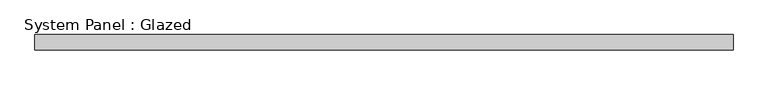
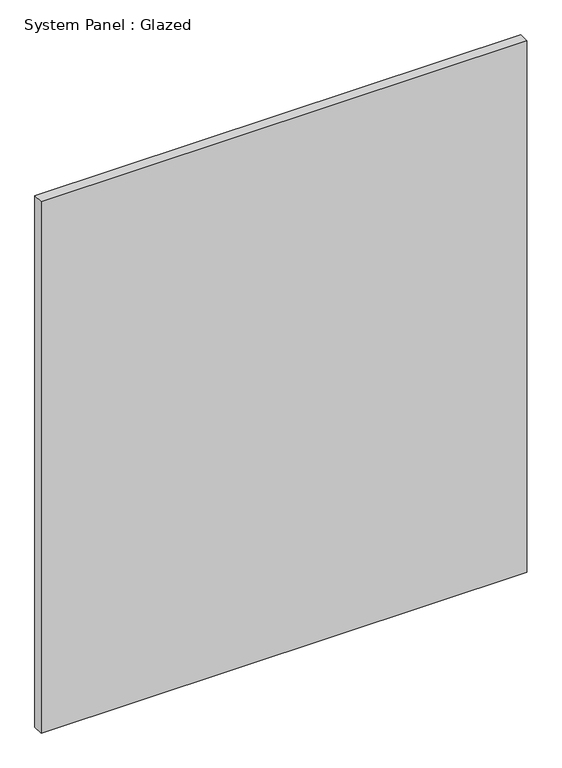
"""IFC4 building model written with IfcOpenShell, lengths in millimetres: plate geometry, System Panel : Glazed."""

from ifc_helpers import new_model, si_unit, origin, origin_with_axes, place, context, project, spatial, polyline, outline, extrude, source, transform, mapped, element, save


def system_panel_glazed_3d395eef(model_context):
    return source(origin(), model_context, "Body", "SweptSolid", [
        extrude(outline(polyline([(575.7333334, 24.5), (-575.7333334, 24.5), (-575.7333334, 49.5), (575.7333334, 49.5), (575.7333334, 24.5)])), origin_with_axes(), (0.0, 0.0, 1.0), 1330.8429687),
    ])


if __name__ == "__main__":
    model = new_model("IFC4")
    model_context = context("Model", 3, world=origin())
    ifc_project = project(units=[si_unit("LENGTHUNIT", "METRE", prefix="MILLI")], contexts=[model_context])
    site = spatial("IfcSite", under=ifc_project)
    building = spatial("IfcBuilding", under=site)
    placement = place(None, origin())
    system_panel_glazed_shape = system_panel_glazed_3d395eef(model_context)
    element("IfcPlate", 1, ObjectType="System Panel : Glazed", at=placement, inside=building, context=model_context, shape_type="MappedRepresentation", body=[
        mapped(system_panel_glazed_shape, transform((0.0, 0.0, 0.0), x_axis=(1.0, 0.0, 0.0), y_axis=(0.0, 1.0, 0.0), z_axis=(0.0, 0.0, 1.0))),
    ])
    save(model, "model.ifc")

# Revit data of these elements
# Type "System Panel : Glazed"
#   Keynote = "H11"
#   Construction Type Id = "GSP4R"
#   Analytic Construction = "1/8 in Pilkington single glazing"
#   Visual Light Transmittance = 0.9
#   Solar Heat Gain Coefficient = 0.86
#   Heat Transfer Coefficient (U) = 6.7069 W/(m²·K)
#   Define Thermal Properties by = 1
# Element 1 (IfcPlate, "System Panel : Glazed")
#   Materials on its faces: "Glass"
# Materials
#   "Glass": class "Glass", colour RGB 0 128 192, transparency 0.9, Description = "Soda Lime Glass", Cost = 0
